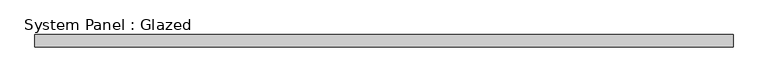
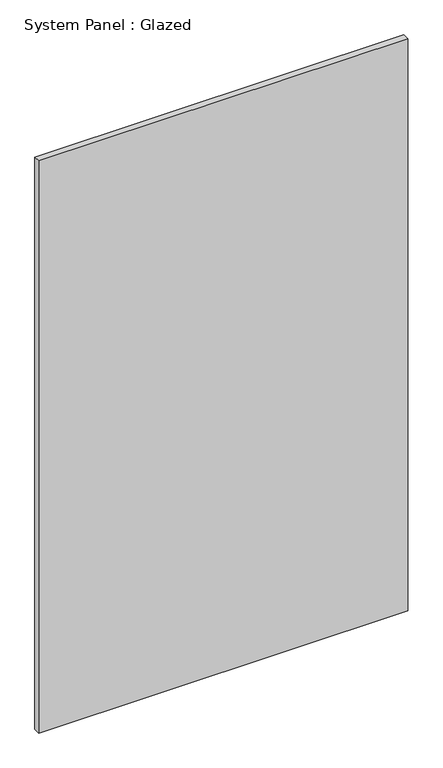
"""IFC4 building model written with IfcOpenShell, lengths in millimetres: plate geometry, System Panel : Glazed."""

from ifc_helpers import new_model, si_unit, origin, origin_with_axes, place, context, project, spatial, polyline, outline, extrude, source, transform, mapped, element, save


def system_panel_glazed_adb83807(model_context):
    return source(origin(), model_context, "Body", "SweptSolid", [
        extrude(outline(polyline([(714.375, -44.45), (-714.375, -44.45), (-714.375, -19.05), (714.375, -19.05), (714.375, -44.45)])), origin_with_axes(), (0.0, 0.0, 1.0), 2343.15),
    ])


if __name__ == "__main__":
    model = new_model("IFC4")
    model_context = context("Model", 3, world=origin())
    ifc_project = project(units=[si_unit("LENGTHUNIT", "METRE", prefix="MILLI")], contexts=[model_context])
    site = spatial("IfcSite", under=ifc_project)
    building = spatial("IfcBuilding", under=site)
    placement = place(None, origin())
    system_panel_glazed_shape = system_panel_glazed_adb83807(model_context)
    element("IfcPlate", 1, ObjectType="System Panel : Glazed", at=placement, inside=building, context=model_context, shape_type="MappedRepresentation", body=[
        mapped(system_panel_glazed_shape, transform((0.0, 0.0, 0.0), x_axis=(1.0, 0.0, 0.0), y_axis=(0.0, 1.0, 0.0), z_axis=(0.0, 0.0, 1.0))),
    ])
    save(model, "model.ifc")

# Revit data of these elements
# Type "System Panel : Glazed"
#   Construction Type Id = "GSP4R"
#   Analytic Construction = "1/8 in Pilkington single glazing"
#   Visual Light Transmittance = 0.9
#   Solar Heat Gain Coefficient = 0.86
#   Heat Transfer Coefficient (U) = 1.18115 BTU/(h·ft²·°F)
# Element 1 (IfcPlate, "System Panel : Glazed")
#   Materials on its faces: "Glass"
# Materials
#   "Glass": class "Glass", colour RGB 0 128 192, transparency 0.75, Description = "Soda Lime Glass", Cost = 0
